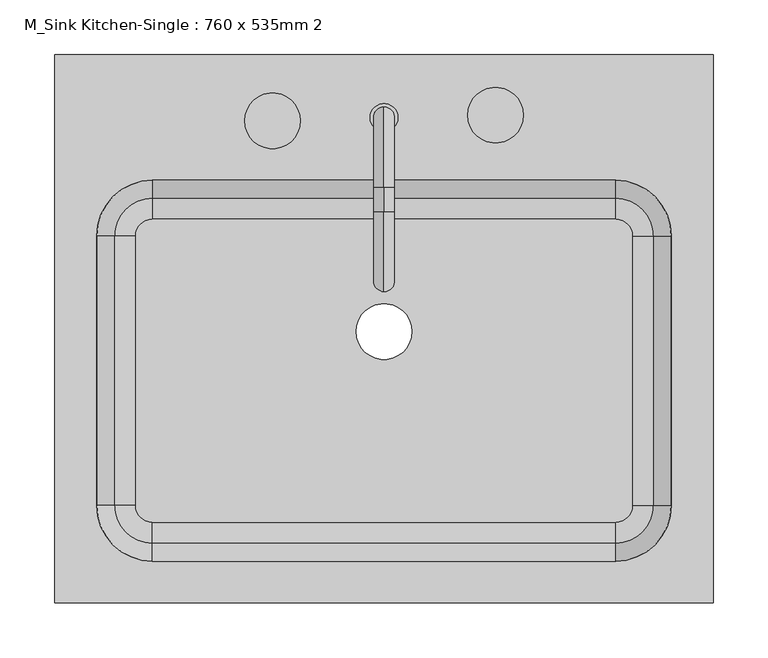
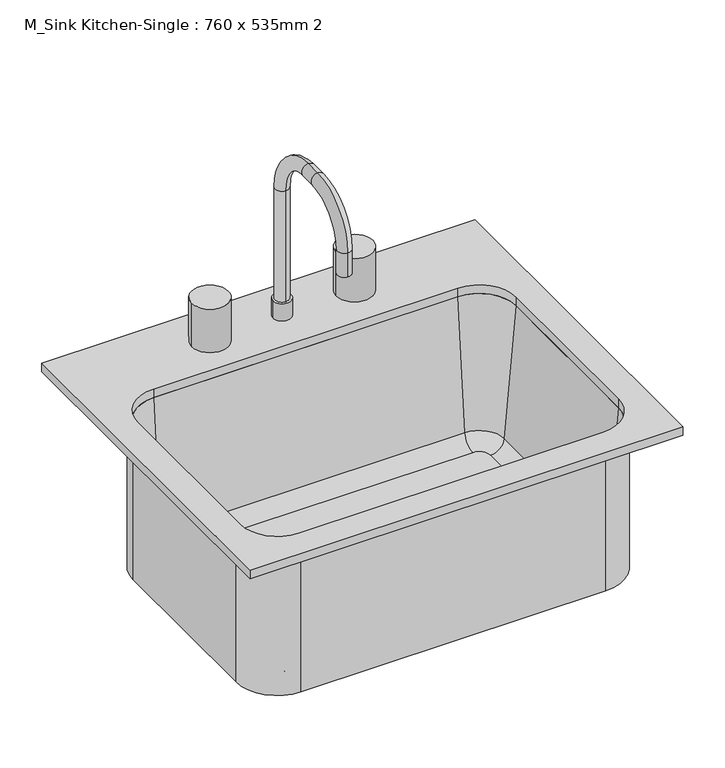
"""IFC4 building model written with IfcOpenShell, lengths in millimetres: flow terminal geometry, M_Sink Kitchen-Single : 760 x 535mm 2."""

from ifc_helpers import new_model, si_unit, point, frame, frame_2d, origin, place, context, project, spatial, polyline, circle_curve, ellipse_curve, trimmed, segment, composite_curve, outline, extrude, source, transform, mapped, element, save
from ifc_brep_helpers import plane_surface, cylinder_surface, revolved_surface, advanced_brep


def m_sink_kitchen_single_760_x_535mm_2_7dd6f654(model_context):
    return source(origin(), model_context, "Body", "SolidModel", [
        advanced_brep(
        [(283.9392406, 87.2454011, 704.1), (226.7892406, 144.3954011, 704.1), (226.7892406, 144.3954011, 920.0), (283.9392406, 87.2454011, 920.0), (283.9392406, -158.7545989, 704.1), (226.7892406, -215.9045989, 704.1), (-195.4107594, -215.9045989, 704.1), (-252.5607594, -158.7545989, 704.1), (-252.5607594, 87.2454011, 704.1), (-195.4107594, 144.3954011, 704.1), (-9.7107594, 0.0, 704.1), (41.0892406, 0.0, 704.1), (242.0776588, 87.2454011, 713.625), (226.7892406, 102.5338193, 713.625), (-195.4107594, 102.5338193, 713.625), (-210.6991776, 87.2454011, 713.625), (-210.6991776, -158.7545989, 713.625), (-195.4107594, -174.0430171, 713.625), (226.7892406, -174.0430171, 713.625), (242.0776588, -158.7545989, 713.625), (-9.7107594, 0.0, 713.625), (41.0892406, 0.0, 713.625), (261.0551678, 87.2454011, 731.0146831), (226.7892406, 121.5113283, 731.0146831), (277.5892406, 87.2454011, 920.0), (226.7892406, 138.0454011, 920.0), (283.9392406, -158.7545989, 920.0), (261.0551678, -158.7545989, 731.0146831), (277.5892406, -158.7545989, 920.0), (226.7892406, -215.9045989, 920.0), (226.7892406, -193.0205261, 731.0146831), (226.7892406, -209.5545989, 920.0), (-195.4107594, -215.9045989, 920.0), (-195.4107594, -193.0205261, 731.0146831), (-195.4107594, -209.5545989, 920.0), (-252.5607594, -158.7545989, 920.0), (-229.6766866, -158.7545989, 731.0146831), (-246.2107594, -158.7545989, 920.0), (-252.5607594, 87.2454011, 920.0), (-229.6766866, 87.2454011, 731.0146831), (-246.2107594, 87.2454011, 920.0), (-195.4107594, 144.3954011, 920.0), (-195.4107594, 121.5113283, 731.0146831), (-195.4107594, 138.0454011, 920.0)],
        [
            (0, 1, circle_curve(frame((226.7892406, 87.2454011, 704.1), z_axis=(0.0, 0.0, 1.0), x_axis=(0.0, 1.0, 0.0)), 57.15)),
            (1, 2),
            (2, 3, circle_curve(frame((226.7892406, 87.2454011, 920.0), z_axis=(0.0, 0.0, -1.0), x_axis=(0.0, 1.0, 0.0)), 57.15)),
            (3, 0),
            (0, 4),
            (4, 5, circle_curve(frame((226.7892406, -158.7545989, 704.1), z_axis=(0.0, 0.0, -1.0), x_axis=(1.0, 0.0, 0.0)), 57.15)),
            (5, 6),
            (6, 7, circle_curve(frame((-195.4107594, -158.7545989, 704.1), z_axis=(0.0, 0.0, -1.0), x_axis=(0.0, -1.0, 0.0)), 57.15)),
            (7, 8),
            (8, 9, circle_curve(frame((-195.4107594, 87.2454011, 704.1), z_axis=(0.0, 0.0, -1.0), x_axis=(-1.0, 0.0, 0.0)), 57.15)),
            (9, 1),
            (10, 11, circle_curve(frame((15.6892406, 0.0, 704.1), z_axis=(0.0, 0.0, 1.0), x_axis=(1.0, 0.0, 0.0)), 25.4)),
            (11, 10, circle_curve(frame((15.6892406, 0.0, 704.1), z_axis=(0.0, 0.0, 1.0), x_axis=(1.0, 0.0, 0.0)), 25.4)),
            (12, 13, circle_curve(frame((226.7892406, 87.2454011, 713.625), z_axis=(0.0, 0.0, 1.0), x_axis=(0.0, 1.0, 0.0)), 15.2884182)),
            (13, 14),
            (14, 15, circle_curve(frame((-195.4107594, 87.2454011, 713.625), z_axis=(0.0, 0.0, 1.0), x_axis=(-1.0, 0.0, 0.0)), 15.2884182)),
            (15, 16),
            (16, 17, circle_curve(frame((-195.4107594, -158.7545989, 713.625), z_axis=(0.0, 0.0, 1.0), x_axis=(0.0, -1.0, 0.0)), 15.2884182)),
            (17, 18),
            (18, 19, circle_curve(frame((226.7892406, -158.7545989, 713.625), z_axis=(0.0, 0.0, 1.0), x_axis=(1.0, 0.0, 0.0)), 15.2884182)),
            (19, 12),
            (20, 21, circle_curve(frame((15.6892406, 0.0, 713.625), z_axis=(0.0, 0.0, -1.0), x_axis=(1.0, 0.0, 0.0)), 25.4)),
            (21, 20, circle_curve(frame((15.6892406, 0.0, 713.625), z_axis=(0.0, 0.0, -1.0), x_axis=(1.0, 0.0, 0.0)), 25.4)),
            (12, 22, circle_curve(frame((242.0776588, 87.2454011, 732.675), z_axis=(0.0, -1.0, 0.0), x_axis=(1.0, 0.0, 0.0)), 19.05)),
            (22, 23, circle_curve(frame((226.7892406, 87.2454011, 731.0146831), z_axis=(0.0, 0.0, 1.0), x_axis=(0.0, 1.0, 0.0)), 34.2659272)),
            (23, 13, circle_curve(frame((226.7892406, 102.5338193, 732.675), z_axis=(-1.0, 0.0, 0.0), x_axis=(0.0, 1.0, 0.0)), 19.05)),
            (22, 24),
            (24, 25, circle_curve(frame((226.7892406, 87.2454011, 920.0), z_axis=(0.0, 0.0, 1.0), x_axis=(0.0, 1.0, 0.0)), 50.8)),
            (25, 23),
            (2, 25),
            (24, 3),
            (3, 26),
            (26, 4),
            (19, 27, circle_curve(frame((242.0776588, -158.7545989, 732.675), z_axis=(0.0, -1.0, 0.0), x_axis=(1.0, 0.0, 0.0)), 19.05)),
            (27, 22),
            (27, 28),
            (28, 24),
            (28, 26),
            (26, 29, circle_curve(frame((226.7892406, -158.7545989, 920.0), z_axis=(0.0, 0.0, -1.0), x_axis=(1.0, 0.0, 0.0)), 57.15)),
            (29, 5),
            (18, 30, circle_curve(frame((226.7892406, -174.0430171, 732.675), z_axis=(-1.0, 0.0, 0.0), x_axis=(0.0, -1.0, 0.0)), 19.05)),
            (30, 27, circle_curve(frame((226.7892406, -158.7545989, 731.0146831), z_axis=(0.0, 0.0, 1.0), x_axis=(1.0, 0.0, 0.0)), 34.2659272)),
            (30, 31),
            (31, 28, circle_curve(frame((226.7892406, -158.7545989, 920.0), z_axis=(0.0, 0.0, 1.0), x_axis=(1.0, 0.0, 0.0)), 50.8)),
            (31, 29),
            (29, 32),
            (32, 6),
            (17, 33, circle_curve(frame((-195.4107594, -174.0430171, 732.675), z_axis=(-1.0, 0.0, 0.0), x_axis=(0.0, -1.0, 0.0)), 19.05)),
            (33, 30),
            (33, 34),
            (34, 31),
            (34, 32),
            (32, 35, circle_curve(frame((-195.4107594, -158.7545989, 920.0), z_axis=(0.0, 0.0, -1.0), x_axis=(0.0, -1.0, 0.0)), 57.15)),
            (35, 7),
            (16, 36, circle_curve(frame((-210.6991776, -158.7545989, 732.675), z_axis=(0.0, 1.0, 0.0), x_axis=(-1.0, 0.0, 0.0)), 19.05)),
            (36, 33, circle_curve(frame((-195.4107594, -158.7545989, 731.0146831), z_axis=(0.0, 0.0, 1.0), x_axis=(0.0, -1.0, 0.0)), 34.2659272)),
            (36, 37),
            (37, 34, circle_curve(frame((-195.4107594, -158.7545989, 920.0), z_axis=(0.0, 0.0, 1.0), x_axis=(0.0, -1.0, 0.0)), 50.8)),
            (37, 35),
            (35, 38),
            (38, 8),
            (15, 39, circle_curve(frame((-210.6991776, 87.2454011, 732.675), z_axis=(0.0, 1.0, 0.0), x_axis=(-1.0, 0.0, 0.0)), 19.05)),
            (39, 36),
            (39, 40),
            (40, 37),
            (40, 38),
            (38, 41, circle_curve(frame((-195.4107594, 87.2454011, 920.0), z_axis=(0.0, 0.0, -1.0), x_axis=(-1.0, 0.0, 0.0)), 57.15)),
            (41, 9),
            (14, 42, circle_curve(frame((-195.4107594, 102.5338193, 732.675), z_axis=(1.0, 0.0, 0.0), x_axis=(0.0, 1.0, 0.0)), 19.05)),
            (42, 39, circle_curve(frame((-195.4107594, 87.2454011, 731.0146831), z_axis=(0.0, 0.0, 1.0), x_axis=(-1.0, 0.0, 0.0)), 34.2659272)),
            (42, 43),
            (43, 40, circle_curve(frame((-195.4107594, 87.2454011, 920.0), z_axis=(0.0, 0.0, 1.0), x_axis=(-1.0, 0.0, 0.0)), 50.8)),
            (43, 41),
            (41, 2),
            (23, 42),
            (25, 43),
            (20, 10),
            (11, 21),
        ],
        [
            cylinder_surface(frame((226.7892406, 87.2454011, 0.0), z_axis=(0.0, 0.0, -1.0), x_axis=(0.0, 1.0, 0.0)), 57.15),
            plane_surface(frame((226.7892406, 87.2454011, 704.1), z_axis=(0.0, 0.0, -1.0), x_axis=(0.0, 1.0, 0.0))),
            plane_surface(frame((226.7892406, 87.2454011, 713.625), z_axis=(0.0, 0.0, 1.0), x_axis=(0.0, 1.0, 0.0))),
            revolved_surface(trimmed(ellipse_curve(frame((226.7892406, 102.5338193, 732.675), z_axis=(1.0, 0.0, 0.0), x_axis=(0.0, 1.0, 0.0)), 19.05, 19.05), [point((226.7892406, 102.5338193, 713.625))], [point((226.7892406, 121.5113283, 731.0146831))], True, "CARTESIAN"), (226.7892406, 87.2454011, 0.0), (0.0, 0.0, -1.0)),
            revolved_surface(polyline([(226.7892406, 121.5113283, 731.0146831), (226.7892406, 138.0454011, 920.0)]), (226.7892406, 87.2454011, 0.0), (0.0, 0.0, -1.0)),
            plane_surface(frame((226.7892406, 87.2454011, 920.0), z_axis=(0.0, 0.0, 1.0), x_axis=(0.0, 1.0, 0.0))),
            plane_surface(frame((283.9392406, 87.2454011, 920.0), z_axis=(1.0, 0.0, 0.0), x_axis=(0.0, -1.0, 0.0))),
            revolved_surface(polyline([(261.1276588, -158.75459890000002, 732.675), (261.1276588, 87.2454011, 732.675)]), (242.0776588, 87.2454011, 732.675), (0.0, -1.0, 0.0)),
            plane_surface(frame((261.0551678, 87.2454011, 731.0146831), z_axis=(-0.9961946980917443, 0.0, 0.08715574274767207), x_axis=(0.0, -1.0, 0.0))),
            plane_surface(frame((277.5892406, 87.2454011, 920.0), z_axis=(0.0, 0.0, 1.0), x_axis=(0.0, -1.0, 0.0))),
            cylinder_surface(frame((226.7892406, -158.7545989, 0.0), z_axis=(0.0, 0.0, -1.0), x_axis=(1.0, 0.0, 0.0)), 57.15),
            revolved_surface(trimmed(ellipse_curve(frame((242.0776588, -158.7545989, 732.675), z_axis=(0.0, -1.0, 0.0), x_axis=(1.0, 0.0, 0.0)), 19.05, 19.05), [point((242.0776588, -158.7545989, 713.625))], [point((261.0551678, -158.7545989, 731.0146831))], True, "CARTESIAN"), (226.7892406, -158.7545989, 0.0), (0.0, 0.0, -1.0)),
            revolved_surface(polyline([(261.0551678, -158.7545989, 731.0146831), (277.5892406, -158.7545989, 920.0)]), (226.7892406, -158.7545989, 0.0), (0.0, 0.0, -1.0)),
            plane_surface(frame((226.7892406, -158.7545989, 920.0), z_axis=(0.0, 0.0, 1.0), x_axis=(1.0, 0.0, 0.0))),
            plane_surface(frame((226.7892406, -215.9045989, 920.0), z_axis=(0.0, -1.0, 0.0), x_axis=(-1.0, 0.0, 0.0))),
            revolved_surface(polyline([(-195.4107594, -193.0930171, 732.675), (226.7892406, -193.0930171, 732.675)]), (226.7892406, -174.0430171, 732.675), (-1.0, 0.0, 0.0)),
            plane_surface(frame((226.7892406, -193.0205261, 731.0146831), z_axis=(0.0, 0.9961946980917443, 0.08715574274767207), x_axis=(-1.0, 0.0, 0.0))),
            plane_surface(frame((226.7892406, -209.5545989, 920.0), z_axis=(0.0, 0.0, 1.0), x_axis=(-1.0, 0.0, 0.0))),
            cylinder_surface(frame((-195.4107594, -158.7545989, 0.0), z_axis=(0.0, 0.0, -1.0), x_axis=(0.0, -1.0, 0.0)), 57.15),
            revolved_surface(trimmed(ellipse_curve(frame((-195.4107594, -174.0430171, 732.675), z_axis=(-1.0, 0.0, 0.0), x_axis=(0.0, -1.0, 0.0)), 19.05, 19.05), [point((-195.4107594, -174.0430171, 713.625))], [point((-195.4107594, -193.0205261, 731.0146831))], True, "CARTESIAN"), (-195.4107594, -158.7545989, 0.0), (0.0, 0.0, -1.0)),
            revolved_surface(polyline([(-195.4107594, -193.0205261, 731.0146831), (-195.4107594, -209.5545989, 920.0)]), (-195.4107594, -158.7545989, 0.0), (0.0, 0.0, -1.0)),
            plane_surface(frame((-195.4107594, -158.7545989, 920.0), z_axis=(0.0, 0.0, 1.0), x_axis=(0.0, -1.0, 0.0))),
            plane_surface(frame((-252.5607594, -158.7545989, 920.0), z_axis=(-1.0, 0.0, 0.0), x_axis=(0.0, 1.0, 0.0))),
            revolved_surface(polyline([(-229.74917760000002, 87.24540110000001, 732.675), (-229.74917760000002, -158.7545989, 732.675)]), (-210.6991776, -158.7545989, 732.675), (0.0, 1.0, 0.0)),
            plane_surface(frame((-229.6766866, -158.7545989, 731.0146831), z_axis=(0.9961946980917443, 0.0, 0.08715574274767207), x_axis=(0.0, 1.0, 0.0))),
            plane_surface(frame((-246.2107594, -158.7545989, 920.0), z_axis=(0.0, 0.0, 1.0), x_axis=(0.0, 1.0, 0.0))),
            cylinder_surface(frame((-195.4107594, 87.2454011, 0.0), z_axis=(0.0, 0.0, -1.0), x_axis=(-1.0, 0.0, 0.0)), 57.15),
            revolved_surface(trimmed(ellipse_curve(frame((-210.6991776, 87.2454011, 732.675), z_axis=(0.0, 1.0, 0.0), x_axis=(-1.0, 0.0, 0.0)), 19.05, 19.05), [point((-210.6991776, 87.2454011, 713.625))], [point((-229.6766866, 87.2454011, 731.0146831))], True, "CARTESIAN"), (-195.4107594, 87.2454011, 0.0), (0.0, 0.0, -1.0)),
            revolved_surface(polyline([(-229.6766866, 87.2454011, 731.0146831), (-246.2107594, 87.2454011, 920.0)]), (-195.4107594, 87.2454011, 0.0), (0.0, 0.0, -1.0)),
            plane_surface(frame((-195.4107594, 87.2454011, 920.0), z_axis=(0.0, 0.0, 1.0), x_axis=(-1.0, 0.0, 0.0))),
            plane_surface(frame((-195.4107594, 144.3954011, 920.0), z_axis=(0.0, 1.0, 0.0), x_axis=(1.0, 0.0, 0.0))),
            revolved_surface(polyline([(226.7892406, 121.5838193, 732.675), (-195.4107594, 121.5838193, 732.675)]), (-195.4107594, 102.5338193, 732.675), (1.0, 0.0, 0.0)),
            plane_surface(frame((-195.4107594, 121.5113283, 731.0146831), z_axis=(0.0, -0.9961946980917443, 0.08715574274767207), x_axis=(1.0, 0.0, 0.0))),
            plane_surface(frame((-195.4107594, 138.0454011, 920.0), z_axis=(0.0, 0.0, 1.0), x_axis=(1.0, 0.0, 0.0))),
            revolved_surface(polyline([(41.0892406, 0.0, 704.1), (41.0892406, 0.0, 713.625)]), (15.6892406, 0.0, 0.0), (0.0, 0.0, -1.0)),
        ],
        [
            (0, [[1, 2, 3, 4]]),
            (1, [[-1, 5, 6, 7, 8, 9, 10, 11], [12, 13]]),
            (2, [[14, 15, 16, 17, 18, 19, 20, 21], [22, 23]]),
            (3, [[-14, 24, 25, 26]]),
            (4, [[-25, 27, 28, 29]]),
            (5, [[-3, 30, -28, 31]]),
            (6, [[-4, 32, 33, -5]]),
            (7, [[-24, -21, 34, 35]]),
            (8, [[-27, -35, 36, 37]]),
            (9, [[-31, -37, 38, -32]]),
            (10, [[-33, 39, 40, -6]]),
            (11, [[-34, -20, 41, 42]]),
            (12, [[-36, -42, 43, 44]]),
            (13, [[-38, -44, 45, -39]]),
            (14, [[-40, 46, 47, -7]]),
            (15, [[-41, -19, 48, 49]]),
            (16, [[-43, -49, 50, 51]]),
            (17, [[-45, -51, 52, -46]]),
            (18, [[-47, 53, 54, -8]]),
            (19, [[-48, -18, 55, 56]]),
            (20, [[-50, -56, 57, 58]]),
            (21, [[-52, -58, 59, -53]]),
            (22, [[-54, 60, 61, -9]]),
            (23, [[-55, -17, 62, 63]]),
            (24, [[-57, -63, 64, 65]]),
            (25, [[-59, -65, 66, -60]]),
            (26, [[-61, 67, 68, -10]]),
            (27, [[-62, -16, 69, 70]]),
            (28, [[-64, -70, 71, 72]]),
            (29, [[-66, -72, 73, -67]]),
            (30, [[-2, -11, -68, 74]]),
            (31, [[-26, 75, -69, -15]]),
            (32, [[-29, 76, -71, -75]]),
            (33, [[-30, -74, -73, -76]]),
            (34, [[-22, 77, -13, 78]]),
            (34, [[-23, -78, -12, -77]]),
        ],
    ),
        advanced_brep(
        [(2.9892406, 195.1954011, 958.1), (28.3892406, 195.1954011, 958.1), (15.6892406, 204.7204011, 958.1), (15.6892406, 185.6704011, 958.1), (2.9892406, 195.1954011, 932.7), (28.3892406, 195.1954011, 932.7), (15.6892406, 204.7204011, 1120.025), (15.6892406, 185.6704011, 1120.025), (15.6892406, 131.6954011, 1193.05), (15.6892406, 131.6954011, 1174.0), (15.6892406, 109.4704011, 1193.05), (15.6892406, 109.4704011, 1174.0), (15.6892406, 36.4454011, 1120.025), (15.6892406, 55.4954011, 1120.025), (15.6892406, 36.4454011, 1085.1), (15.6892406, 55.4954011, 1085.1)],
        [
            (0, 1, circle_curve(frame((15.6892406, 195.1954011, 958.1), z_axis=(0.0, 0.0, 1.0), x_axis=(1.0, 0.0, 0.0)), 12.7)),
            (1, 0, circle_curve(frame((15.6892406, 195.1954011, 958.1), z_axis=(0.0, 0.0, 1.0), x_axis=(1.0, 0.0, 0.0)), 12.7)),
            (2, 3, circle_curve(frame((15.6892406, 195.1954011, 958.1), z_axis=(0.0, 0.0, -1.0), x_axis=(0.0, -1.0, 0.0)), 9.525)),
            (3, 2, circle_curve(frame((15.6892406, 195.1954011, 958.1), z_axis=(0.0, 0.0, -1.0), x_axis=(0.0, -1.0, 0.0)), 9.525)),
            (4, 5, circle_curve(frame((15.6892406, 195.1954011, 932.7), z_axis=(0.0, 0.0, -1.0), x_axis=(1.0, 0.0, 0.0)), 12.7)),
            (5, 4, circle_curve(frame((15.6892406, 195.1954011, 932.7), z_axis=(0.0, 0.0, -1.0), x_axis=(1.0, 0.0, 0.0)), 12.7)),
            (0, 4),
            (5, 1),
            (6, 7, circle_curve(frame((15.6892406, 195.1954011, 1120.025), z_axis=(0.0, 0.0, -1.0), x_axis=(0.0, -1.0, 0.0)), 9.525)),
            (7, 3),
            (2, 6),
            (7, 6, circle_curve(frame((15.6892406, 195.1954011, 1120.025), z_axis=(0.0, 0.0, -1.0), x_axis=(0.0, -1.0, 0.0)), 9.525)),
            (6, 8, circle_curve(frame((15.6892406, 131.6954011, 1120.025), z_axis=(1.0, 0.0, 0.0), x_axis=(0.0, 1.0, 0.0)), 73.025)),
            (8, 9, circle_curve(frame((15.6892406, 131.6954011, 1183.525), z_axis=(0.0, 1.0, 0.0), x_axis=(0.0, 0.0, -1.0)), 9.525)),
            (9, 7, circle_curve(frame((15.6892406, 131.6954011, 1120.025), z_axis=(-1.0, 0.0, 0.0), x_axis=(0.0, 1.0, 0.0)), 53.975)),
            (9, 8, circle_curve(frame((15.6892406, 131.6954011, 1183.525), z_axis=(0.0, 1.0, 0.0), x_axis=(0.0, 0.0, -1.0)), 9.525)),
            (8, 10),
            (10, 11, circle_curve(frame((15.6892406, 109.4704011, 1183.525), z_axis=(0.0, 1.0, 0.0), x_axis=(0.0, 0.0, -1.0)), 9.525)),
            (11, 9),
            (11, 10, circle_curve(frame((15.6892406, 109.4704011, 1183.525), z_axis=(0.0, 1.0, 0.0), x_axis=(0.0, 0.0, -1.0)), 9.525)),
            (10, 12, circle_curve(frame((15.6892406, 109.4704011, 1120.025), z_axis=(1.0, 0.0, 0.0), x_axis=(0.0, 0.0, 1.0)), 73.025)),
            (12, 13, circle_curve(frame((15.6892406, 45.9704011, 1120.025), z_axis=(0.0, 0.0, 1.0), x_axis=(0.0, 1.0, 0.0)), 9.525)),
            (13, 11, circle_curve(frame((15.6892406, 109.4704011, 1120.025), z_axis=(-1.0, 0.0, 0.0), x_axis=(0.0, 0.0, 1.0)), 53.975)),
            (13, 12, circle_curve(frame((15.6892406, 45.9704011, 1120.025), z_axis=(0.0, 0.0, 1.0), x_axis=(0.0, 1.0, 0.0)), 9.525)),
            (14, 15, circle_curve(frame((15.6892406, 45.9704011, 1085.1), z_axis=(0.0, 0.0, -1.0), x_axis=(0.0, 1.0, 0.0)), 9.525)),
            (15, 14, circle_curve(frame((15.6892406, 45.9704011, 1085.1), z_axis=(0.0, 0.0, -1.0), x_axis=(0.0, 1.0, 0.0)), 9.525)),
            (12, 14),
            (15, 13),
        ],
        [
            plane_surface(frame((28.3892406, 195.1954011, 958.1), z_axis=(0.0, 0.0, 1.0), x_axis=(0.0, 1.0, 0.0))),
            plane_surface(frame((28.3892406, 195.1954011, 932.7), z_axis=(0.0, 0.0, -1.0), x_axis=(0.0, -1.0, 0.0))),
            cylinder_surface(frame((15.6892406, 195.1954011, 932.7), z_axis=(0.0, 0.0, 1.0), x_axis=(1.0, 0.0, 0.0)), 12.7),
            cylinder_surface(frame((15.6892406, 195.1954011, 932.7), z_axis=(0.0, 0.0, -1.0), x_axis=(0.0, -1.0, 0.0)), 9.525),
            revolved_surface(trimmed(ellipse_curve(frame((15.6892406, 195.1954011, 1120.025), z_axis=(0.0, 0.0, -1.0), x_axis=(0.0, -1.0, 0.0)), 9.525, 9.525), [point((15.6892406, 204.7204011, 1120.025))], [point((15.6892406, 185.6704011, 1120.025))], True, "CARTESIAN"), (15.6892406, 131.6954011, 1120.025), (1.0, 0.0, 0.0)),
            revolved_surface(trimmed(ellipse_curve(frame((15.6892406, 195.1954011, 1120.025), z_axis=(0.0, 0.0, -1.0), x_axis=(0.0, -1.0, 0.0)), 9.525, 9.525), [point((15.6892406, 185.6704011, 1120.025))], [point((15.6892406, 204.7204011, 1120.025))], True, "CARTESIAN"), (15.6892406, 131.6954011, 1120.025), (1.0, 0.0, 0.0)),
            cylinder_surface(frame((15.6892406, 131.6954011, 1183.525), z_axis=(0.0, 1.0, 0.0), x_axis=(0.0, 0.0, -1.0)), 9.525),
            revolved_surface(trimmed(ellipse_curve(frame((15.6892406, 109.4704011, 1183.525), z_axis=(0.0, 1.0, 0.0), x_axis=(0.0, 0.0, -1.0)), 9.525, 9.525), [point((15.6892406, 109.4704011, 1193.05))], [point((15.6892406, 109.4704011, 1174.0))], True, "CARTESIAN"), (15.6892406, 109.4704011, 1120.025), (1.0, 0.0, 0.0)),
            revolved_surface(trimmed(ellipse_curve(frame((15.6892406, 109.4704011, 1183.525), z_axis=(0.0, 1.0, 0.0), x_axis=(0.0, 0.0, -1.0)), 9.525, 9.525), [point((15.6892406, 109.4704011, 1174.0))], [point((15.6892406, 109.4704011, 1193.05))], True, "CARTESIAN"), (15.6892406, 109.4704011, 1120.025), (1.0, 0.0, 0.0)),
            plane_surface(frame((15.6892406, 36.4454011, 1085.1), z_axis=(0.0, 0.0, -1.0), x_axis=(-1.0, 0.0, 0.0))),
            cylinder_surface(frame((15.6892406, 45.9704011, 1120.025), z_axis=(0.0, 0.0, 1.0), x_axis=(0.0, 1.0, 0.0)), 9.525),
        ],
        [
            (0, [[1, 2], [3, 4]]),
            (1, [[5, 6]]),
            (2, [[-1, 7, -6, 8]]),
            (2, [[-2, -8, -5, -7]]),
            (3, [[9, 10, -3, 11]]),
            (3, [[12, -11, -4, -10]]),
            (4, [[-9, 13, 14, 15]]),
            (5, [[-12, -15, 16, -13]]),
            (6, [[-14, 17, 18, 19]]),
            (6, [[-16, -19, 20, -17]]),
            (7, [[-18, 21, 22, 23]]),
            (8, [[-20, -23, 24, -21]]),
            (9, [[25, 26]]),
            (10, [[-22, 27, -26, 28]]),
            (10, [[-24, -28, -25, -27]]),
        ],
    ),
        extrude(outline(composite_curve([segment(trimmed(circle_curve(frame_2d((-85.9107594, 192.1166076)), 25.4), [point((-111.3107594, 192.1166076))], [point((-60.5107594, 192.1166076))], False, "CARTESIAN"), True, "CONTINUOUS"), segment(trimmed(circle_curve(frame_2d((-85.9107594, 192.1166076)), 25.4), [point((-60.5107594, 192.1166076))], [point((-111.3107594, 192.1166076))], False, "CARTESIAN"), True, "CONTINUOUS")], self_intersect=False)), frame((0.0, 0.0, 932.7), z_axis=(0.0, 0.0, 1.0), x_axis=(1.0, 0.0, 0.0)), (0.0, 0.0, 1.0), 63.5),
        extrude(outline(composite_curve([segment(trimmed(circle_curve(frame_2d((117.2892406, 197.3133323)), 25.4), [point((91.8892406, 197.3133323))], [point((142.6892406, 197.3133323))], False, "CARTESIAN"), True, "CONTINUOUS"), segment(trimmed(circle_curve(frame_2d((117.2892406, 197.3133323)), 25.4), [point((142.6892406, 197.3133323))], [point((91.8892406, 197.3133323))], False, "CARTESIAN"), True, "CONTINUOUS")], self_intersect=False)), frame((0.0, 0.0, 932.7), z_axis=(0.0, 0.0, 1.0), x_axis=(1.0, 0.0, 0.0)), (0.0, 0.0, 1.0), 63.5),
        extrude(outline(polyline([(315.6892406, 252.3454011), (315.6892406, -247.6545989), (-284.3107594, -247.6545989), (-284.3107594, 252.3454011), (315.6892406, 252.3454011)]), holes=[composite_curve([segment(polyline([(226.7892406, 138.0454011), (-195.4107594, 138.0454011)]), True, "CONTINUOUS"), segment(trimmed(circle_curve(frame_2d((-195.4107594, 87.2454011)), 50.8), [point((-195.4107594, 138.0454011))], [point((-246.2107594, 87.2454011))], True, "CARTESIAN"), True, "CONTINUOUS"), segment(polyline([(-246.2107594, 87.2454011), (-246.2107594, -158.7545989)]), True, "CONTINUOUS"), segment(trimmed(circle_curve(frame_2d((-195.4107594, -158.7545989)), 50.8), [point((-246.2107594, -158.7545989))], [point((-195.4107594, -209.5545989))], True, "CARTESIAN"), True, "CONTINUOUS"), segment(polyline([(-195.4107594, -209.5545989), (226.7892406, -209.5545989)]), True, "CONTINUOUS"), segment(trimmed(circle_curve(frame_2d((226.7892406, -158.7545989)), 50.8), [point((226.7892406, -209.5545989))], [point((277.5892406, -158.7545989))], True, "CARTESIAN"), True, "CONTINUOUS"), segment(polyline([(277.5892406, -158.7545989), (277.5892406, 87.2454011)]), True, "CONTINUOUS"), segment(trimmed(circle_curve(frame_2d((226.7892406, 87.2454011)), 50.8), [point((277.5892406, 87.2454011))], [point((226.7892406, 138.0454011))], True, "CARTESIAN"), True, "CONTINUOUS")], self_intersect=False)]), frame((0.0, 0.0, 920.0), z_axis=(0.0, 0.0, 1.0), x_axis=(1.0, 0.0, 0.0)), (0.0, 0.0, 1.0), 12.7),
    ])


if __name__ == "__main__":
    model = new_model("IFC4")
    model_context = context("Model", 3, world=origin())
    ifc_project = project(units=[si_unit("LENGTHUNIT", "METRE", prefix="MILLI")], contexts=[model_context])
    site = spatial("IfcSite", under=ifc_project)
    building = spatial("IfcBuilding", under=site)
    placement = place(None, origin())
    m_sink_kitchen_single_760_x_535mm_2_shape = m_sink_kitchen_single_760_x_535mm_2_7dd6f654(model_context)
    element("IfcFlowTerminal", 1, ObjectType="M_Sink Kitchen-Single : 760 x 535mm 2", at=placement, inside=building, context=model_context, shape_type="MappedRepresentation", body=[
        mapped(m_sink_kitchen_single_760_x_535mm_2_shape, transform((0.0, 0.0, 0.0), x_axis=(1.0, 0.0, 0.0), y_axis=(0.0, 1.0, 0.0), z_axis=(0.0, 0.0, 1.0))),
    ])
    save(model, "model.ifc")

# Revit data of these elements
# Type "M_Sink Kitchen-Single : 760 x 535mm 2"
#   Counter Height = 3' - 0.22047"
#   Depth = 1' - 7.68504"
#   Width = 1' - 11.62205"
#   Fixture Material = Metal - Steel, Polished
#   Sink Material = Metal - Steel, Polished
#   Default Elevation = 0
#   Assembly Code = ""
# Element 1 (IfcFlowTerminal, "M_Sink Kitchen-Single : 760 x 535mm 2")
#   Materials on its faces: "Metal - Steel, Polished"
# Materials
#   "Metal - Steel, Polished": class "Metal", colour RGB 192 192 192, transparency 0
